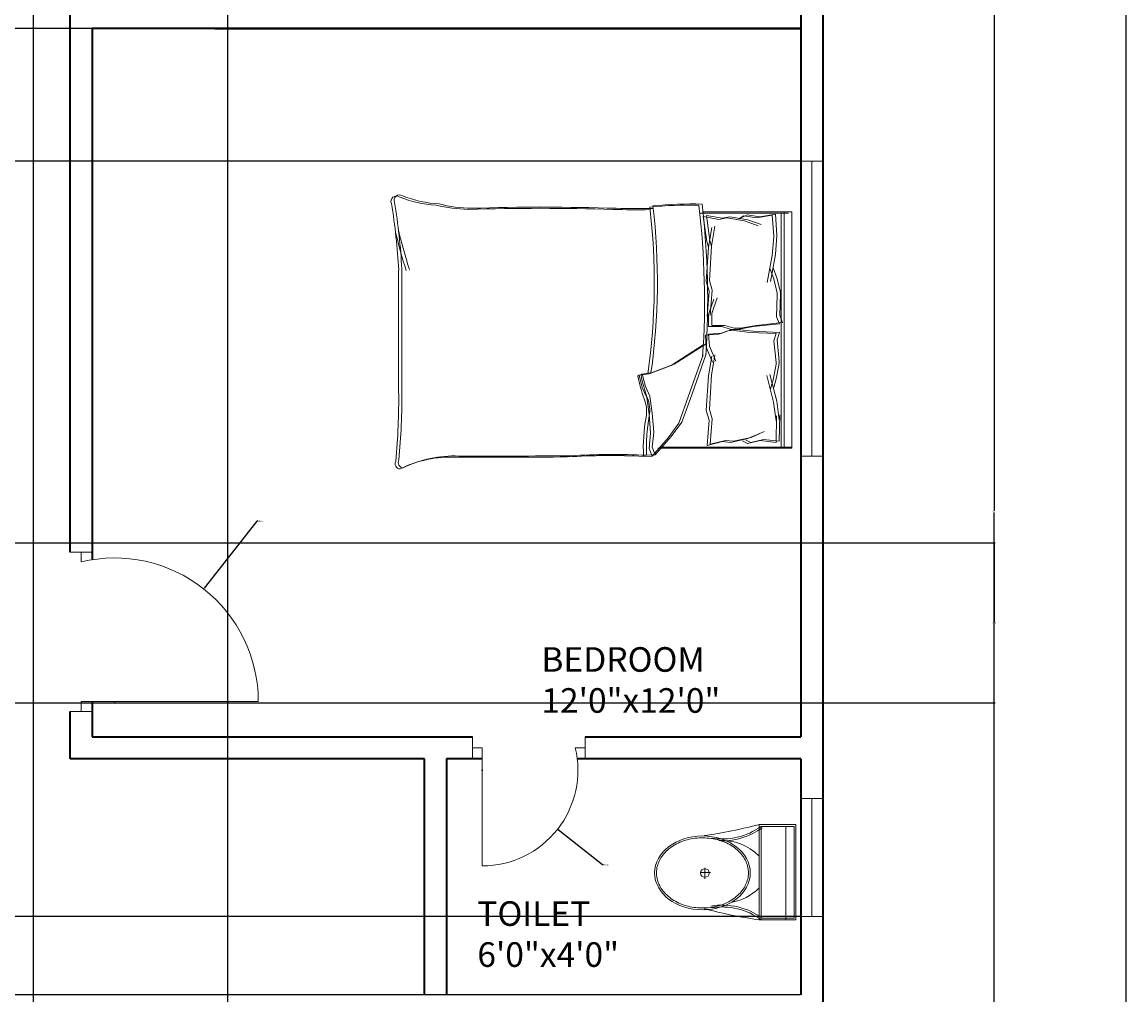
# Model space of a CAD drawing. Units: inches. Extents: x 1861 to 2564, y 1482 to 2317.
# Tile 9 of 11: x 2339 to 2564, y 1853 to 2051. Entities that reach past the tile are written whole.
import ezdxf

# ---------------------------------------------------------------- set-up
doc = ezdxf.new("R2010")
doc.units = ezdxf.units.IN
for name, color, linetype, lineweight in [('A-ANNO-DIMS', 2, 'Continuous', 18), ('A-ANNO-TTLB', 7, 'Continuous', 25), ('A-AREA-IDEN', 7, 'Continuous', 18), ('A-DOOR', 3, 'Continuous', 18), ('A-FLOR-FIXT', 8, 'Continuous', 18), ('A-FURN', 8, 'Continuous', 13), ('A-GLAZ', 4, 'Continuous', 18), ('A-WALL', 7, 'Continuous', 35)]:
    doc.layers.add(name, color=color, linetype=linetype, lineweight=lineweight)
doc.styles.get("Standard").update_dxf_attribs({"font": 'arial.ttf'})
doc.dimstyles.get("Standard").update_dxf_attribs({"dimtxt": 0.18, "dimasz": 0.18, "dimexe": 0.18, "dimexo": 0.0625, "dimgap": 0.09, "dimtad": 0, "dimtih": 1, "dimtoh": 1, "dimdec": 4, "dimzin": 0, "dimdsep": 46, "dimtxsty": 'Standard', "dimcen": 0.09, "dimadec": 0, "dimazin": 0, "dimtfac": 1, "dimtdec": 4, "dimtofl": 0, "dimtmove": 0, "dimatfit": 3, "dimfxl": 1, "dimtolj": 1, "dimtzin": 0, "dimarcsym": 0})

# ---------------------------------------------------------------- blocks, each defined once
blk = doc.blocks.new('A$C31115884')
for p, q in [((283.1, 497.7), (223.4, 497.7)), ((257.5, 466.4), (257.5, 523.2)), ((0, 200), (0, 0)), ((520, 200), (0, 200)), ((10, 190), (10, 10)), ((510, 190), (10, 190)), ((510, 10), (510, 190)), ((520, 0), (520, 200)), ((510, 54.5), (0, 54.5)), ((10, 10), (510, 10)), ((0, 0), (520, 0))]:
    blk.add_line(p, q)
blk.add_circle((255.6, 496.4), 23.6)
for centre, radius, start, end in [((2777.7, -204.6), 2807, 165.4549, 171.71327), ((3237, 905), 2807, 188.28673, 194.5451), ((-294.5, 403.3), 364.7, 324.20913, 9.34987), ((-294.5, 403.3), 374.7, 324.20913, 9.34987), ((805.8, 403.3), 364.7, 170.65013, 215.79087), ((139.5, 406.2), 293.5, 315.84364, 2.65635), ((805.8, 403.3), 374.7, 179.20365, 215.79087), ((383.6, 406.2), 293.5, 190.27735, 224.15636)]:
    blk.add_arc(centre, radius, start, end)
blk.add_ellipse((256.2, 509.9), major_axis=(0, -260.7), ratio=0.772727)
blk.add_open_spline([(256.2, 259.2), (263.1, 259.2), (270, 259.7), (287.8, 262.3), (298.7, 265.1), (319.9, 273.1), (330.2, 278.4), (350.1, 291.1), (359.7, 298.7), (377.7, 315.9), (386.2, 325.5), (401.7, 346.6), (408.8, 358.1), (421.3, 382.5), (426.8, 395.5), (435.9, 422.4), (439.5, 436.4), (444.8, 465.1), (446.5, 479.7), (447.9, 509.2), (447.6, 524), (445, 553.3), (442.7, 567.8), (436.3, 596), (432.1, 609.7), (421.9, 636), (416, 648.6), (402.5, 672.1), (395, 683), (378.6, 703), (369.8, 712.1), (351.1, 728), (341.3, 734.8), (320.9, 746.2), (310.4, 750.7), (288.9, 757.3), (278, 759.4), (256, 761), (245, 760.6), (223.1, 757.2), (212.3, 754.3), (191.1, 746.1), (180.8, 740.7), (160.9, 727.8), (151.4, 720.1), (133.5, 702.7), (125.1, 693), (109.6, 671.7), (102.6, 660.2), (90.2, 635.7), (84.9, 622.7), (76, 595.6), (72.4, 581.6), (67.2, 552.9), (65.6, 538.2), (64.4, 508.8), (64.8, 494), (67.5, 464.7), (69.9, 450.2), (76.6, 422), (80.8, 408.3), (91.1, 382.2), (97.2, 369.7), (110.8, 346.3), (118.4, 335.4), (134.8, 315.6), (143.7, 306.7), (162.4, 290.9), (172.3, 284.2), (192.8, 273), (203.3, 268.6), (224.8, 262.2), (235.8, 260.2), (249.9, 259.3), (253, 259.2), (256.2, 259.2)], degree=3, knots=[0, 0, 0, 0, 0.110105, 0.110105, 0.285049, 0.285049, 0.459994, 0.459994, 0.634938, 0.634938, 0.809882, 0.809882, 0.984827, 0.984827, 1.159771, 1.159771, 1.334715, 1.334715, 1.50966, 1.50966, 1.684604, 1.684604, 1.859549, 1.859549, 2.034493, 2.034493, 2.209437, 2.209437, 2.384382, 2.384382, 2.559326, 2.559326, 2.73427, 2.73427, 2.909215, 2.909215, 3.084159, 3.084159, 3.259103, 3.259103, 3.434048, 3.434048, 3.608992, 3.608992, 3.783936, 3.783936, 3.958881, 3.958881, 4.133825, 4.133825, 4.30877, 4.30877, 4.483714, 4.483714, 4.658658, 4.658658, 4.833603, 4.833603, 5.008547, 5.008547, 5.183491, 5.183491, 5.358436, 5.358436, 5.53338, 5.53338, 5.708324, 5.708324, 5.883269, 5.883269, 6.058213, 6.058213, 6.233158, 6.233158, 6.283185, 6.283185, 6.283185, 6.283185])
blk = doc.blocks.new('WIN-24IN')
for p, q in [((0, 24), (4.5, 24)), ((4.5, 24), (2.25, 24)), ((2.25, 24), (2.25, 0)), ((2.25, 0), (0, 0)), ((0, 0), (4.5, 0))]:
    blk.add_line(p, q)
blk = doc.blocks.new('WIN-60IN')
for p, q in [((0, 4.5), (0, 0)), ((60, 2.25), (60, 4.5)), ((60, 4.5), (60, 0)), ((0, 0), (0, 2.25)), ((0, 2.25), (60, 2.25))]:
    blk.add_line(p, q)
blk = doc.blocks.new('BED-DOUBLE')
for p, q in [((3.48, 63.34), (3.48, 81.45)), ((3.48, 63.34), (3.48, 81.45)), ((51.27, 81.45), (3.48, 81.45)), ((3.7, 62.7), (3.7, 80.81)), ((3.7, 62.7), (3.7, 80.81)), ((51.27, 81.45), (51.27, 54.84)), ((51.27, 81.45), (51.27, 54.84)), ((51.27, 81.45), (51.49, 81.45)), ((51.49, 81.45), (51.49, 80.81)), ((51.49, 80.81), (51.49, 54.2)), ((51.49, 80.81), (51.49, 54.2)), ((3.48, 79.91), (51.27, 79.91)), ((3.48, 79.91), (51.27, 79.91)), ((3.7, 79.27), (51.49, 79.27)), ((3.7, 79.27), (51.49, 79.27)), ((16.88, 78.42), (19.77, 79.14)), ((16.88, 78.42), (19.77, 79.14)), ((19.77, 79.14), (20.09, 79.14)), ((19.77, 79.14), (20.09, 79.14)), ((20.09, 79.14), (24.54, 79)), ((20.09, 79.14), (24.54, 79)), ((24.54, 79), (25.98, 79.58)), ((24.54, 79), (25.98, 79.58)), ((24.77, 78.36), (26.21, 78.94)), ((24.77, 78.36), (26.21, 78.94)), ((25.98, 79.58), (26.56, 74.23)), ((25.98, 79.58), (26.56, 74.23)), ((26.21, 78.94), (26.79, 73.59)), ((26.21, 78.94), (26.79, 73.59)), ((27.98, 78.95), (27.73, 73.58)), ((27.98, 78.95), (27.73, 73.58)), ((29.46, 78.47), (27.98, 78.95)), ((29.46, 78.47), (27.98, 78.95)), ((33.88, 78.89), (29.46, 78.47)), ((33.88, 78.89), (29.46, 78.47)), ((34.21, 78.91), (33.88, 78.89)), ((34.21, 78.91), (33.88, 78.89)), ((37.14, 78.37), (34.21, 78.91)), ((37.14, 78.37), (34.21, 78.91)), ((45.71, 78.9), (41.92, 78.38)), ((45.71, 78.9), (41.92, 78.38)), ((50.11, 78.89), (44.71, 78.99)), ((44.71, 78.99), (45.71, 78.9)), ((50.11, 78.89), (44.71, 78.99)), ((44.71, 78.99), (45.71, 78.9)), ((50.11, 78.89), (49.73, 75.68)), ((50.11, 78.89), (49.73, 75.68)), ((3.9, 78.11), (8.18, 78.44)), ((3.9, 78.11), (8.18, 78.44)), ((3.9, 78.13), (4.47, 74.95)), ((3.9, 78.13), (4.47, 74.95)), ((4.12, 77.49), (4.7, 74.31)), ((4.12, 77.49), (4.7, 74.31)), ((4.13, 77.47), (8.41, 77.8)), ((4.13, 77.47), (8.41, 77.8)), ((8.18, 78.44), (8.29, 78.42)), ((8.18, 78.44), (8.29, 78.42)), ((8.29, 78.42), (12.11, 78.13)), ((8.29, 78.42), (12.11, 78.13)), ((8.41, 77.8), (8.51, 77.78)), ((8.41, 77.8), (8.51, 77.78)), ((8.51, 77.78), (12.34, 77.49)), ((8.51, 77.78), (12.34, 77.49)), ((12.11, 78.13), (17.6, 77.12)), ((12.11, 78.13), (17.6, 77.12)), ((12.34, 77.49), (17.83, 76.48)), ((12.34, 77.49), (17.83, 76.48)), ((14.86, 77.7), (16.88, 78.42)), ((14.86, 77.7), (16.88, 78.42)), ((15.08, 77.06), (17.11, 77.78)), ((15.08, 77.06), (17.11, 77.78)), ((17.11, 77.78), (20, 78.5)), ((17.11, 77.78), (20, 78.5)), ((20, 78.5), (20.32, 78.5)), ((20, 78.5), (20.32, 78.5)), ((20.32, 78.5), (24.77, 78.36)), ((20.32, 78.5), (24.77, 78.36)), ((28.21, 78.31), (27.96, 72.94)), ((28.21, 78.31), (27.96, 72.94)), ((29.69, 77.83), (28.21, 78.31)), ((29.68, 77.83), (28.21, 78.31)), ((34.11, 78.25), (29.68, 77.83)), ((34.11, 78.25), (29.69, 77.83)), ((34.43, 78.27), (34.11, 78.25)), ((34.43, 78.27), (34.11, 78.25)), ((37.36, 77.73), (34.43, 78.27)), ((37.36, 77.73), (34.43, 78.27)), ((41.92, 78.38), (36.5, 77.02)), ((41.92, 78.38), (36.5, 77.02)), ((42.14, 77.74), (36.72, 76.38)), ((42.14, 77.74), (36.72, 76.38)), ((39.2, 77.77), (37.14, 78.37)), ((39.2, 77.77), (37.14, 78.37)), ((39.43, 77.13), (37.36, 77.73)), ((39.43, 77.13), (37.36, 77.73)), ((45.94, 78.26), (42.14, 77.74)), ((45.94, 78.26), (42.14, 77.74)), ((50.34, 78.25), (44.94, 78.35)), ((44.94, 78.35), (45.94, 78.26)), ((50.34, 78.25), (44.94, 78.35)), ((44.94, 78.35), (45.94, 78.26)), ((50.34, 78.25), (49.96, 75.04)), ((50.34, 78.25), (49.96, 75.04)), ((4.47, 74.95), (4.04, 72.35)), ((4.47, 74.95), (4.04, 72.35)), ((4.7, 74.31), (4.27, 71.71)), ((4.7, 74.31), (4.27, 71.71)), ((5.05, 72.49), (6.06, 75.24)), ((5.05, 72.49), (6.06, 75.24)), ((5.28, 71.85), (6.29, 74.6)), ((5.28, 71.85), (6.29, 74.6)), ((26.56, 74.23), (27.14, 71.04)), ((26.56, 74.23), (27.14, 71.04)), ((49.31, 73.19), (48.13, 75.87)), ((49.31, 73.19), (48.13, 75.87)), ((49.54, 72.55), (48.36, 75.23)), ((49.54, 72.55), (48.36, 75.23)), ((49.73, 75.68), (50.33, 73.11)), ((49.73, 75.68), (50.33, 73.11)), ((49.96, 75.04), (50.56, 72.47)), ((49.96, 75.04), (50.56, 72.47)), ((4.04, 72.35), (4.62, 71.33)), ((4.04, 72.35), (4.62, 71.33)), ((4.47, 68.88), (5.05, 72.49)), ((4.47, 68.88), (5.05, 72.49)), ((4.7, 68.24), (5.28, 71.85)), ((4.7, 68.24), (5.28, 71.85)), ((26.79, 73.59), (27.37, 70.41)), ((26.79, 73.59), (27.37, 70.41)), ((27.73, 73.58), (27.36, 70.37)), ((27.73, 73.58), (27.36, 70.37)), ((27.96, 72.94), (27.58, 69.73)), ((27.96, 72.94), (27.58, 69.73)), ((50.11, 69.62), (49.31, 73.19)), ((50.11, 69.62), (49.31, 73.19)), ((50.34, 68.98), (49.54, 72.55)), ((50.34, 68.98), (49.54, 72.55)), ((50.33, 73.11), (49.82, 72.06)), ((50.33, 73.11), (49.82, 72.06)), ((50.56, 72.47), (50.04, 71.42)), ((50.56, 72.47), (50.04, 71.42)), ((4.27, 71.71), (4.85, 70.69)), ((4.27, 71.71), (4.85, 70.69)), ((27.14, 69.74), (26.56, 67.86)), ((27.14, 69.74), (26.56, 67.86)), ((27.14, 71.04), (27.14, 69.74)), ((27.14, 71.04), (27.14, 69.74)), ((27.36, 70.37), (27.44, 69.07)), ((27.36, 70.37), (27.44, 69.07)), ((27.37, 70.41), (27.37, 69.1)), ((27.37, 70.41), (27.37, 69.1)), ((27.58, 69.73), (27.67, 68.43)), ((27.58, 69.73), (27.67, 68.43)), ((49.92, 68.01), (50.11, 69.62)), ((49.92, 68.01), (50.11, 69.62)), ((4.76, 67.29), (4.47, 68.88)), ((4.76, 67.29), (4.47, 68.88)), ((4.99, 66.65), (4.7, 68.24)), ((4.99, 66.65), (4.7, 68.24)), ((26.56, 67.86), (26.56, 65.18)), ((26.56, 67.86), (26.56, 65.18)), ((27.37, 69.1), (26.79, 67.22)), ((27.37, 69.1), (26.79, 67.22)), ((27.44, 69.07), (28.13, 67.23)), ((27.44, 69.07), (28.13, 67.23)), ((27.67, 68.43), (28.36, 66.59)), ((27.67, 68.43), (28.36, 66.59)), ((50.7, 64.87), (49.92, 68.01)), ((50.7, 64.87), (49.92, 68.01)), ((50.15, 67.37), (50.34, 68.98)), ((50.15, 67.37), (50.34, 68.98)), ((50.93, 64.23), (50.15, 67.37)), ((50.93, 64.23), (50.15, 67.37)), ((4.18, 64.1), (4.76, 67.29)), ((4.18, 64.1), (4.76, 67.29)), ((4.41, 63.46), (4.99, 66.65)), ((4.41, 63.46), (4.99, 66.65)), ((6.38, 65.82), (10.41, 65.15)), ((6.38, 65.82), (10.41, 65.15)), ((6.61, 65.18), (10.64, 64.51)), ((6.61, 65.18), (10.64, 64.51)), ((10.41, 65.15), (9.28, 64.83)), ((10.41, 65.15), (9.28, 64.83)), ((10.41, 65.15), (17.42, 64.72)), ((10.41, 65.15), (17.42, 64.72)), ((17.42, 64.72), (19.38, 65.28)), ((17.42, 64.72), (19.38, 65.28)), ((19.38, 65.28), (24.52, 64.87)), ((19.38, 65.28), (24.52, 64.87)), ((24.1, 65.18), (20.96, 66.27)), ((24.1, 65.18), (20.96, 66.27)), ((24.33, 64.54), (21.19, 65.63)), ((24.33, 64.54), (21.19, 65.63)), ((26.56, 65.18), (24.1, 65.18)), ((26.56, 65.18), (24.1, 65.18)), ((26.79, 67.22), (26.79, 64.54)), ((26.79, 67.22), (26.79, 64.54)), ((28.13, 67.23), (28.3, 64.55)), ((28.13, 67.23), (28.3, 64.55)), ((28.36, 66.59), (28.53, 63.91)), ((28.36, 66.59), (28.53, 63.91)), ((30.75, 64.71), (33.82, 65.99)), ((30.75, 64.71), (33.82, 65.99)), ((30.98, 64.07), (34.05, 65.35)), ((30.98, 64.07), (34.05, 65.35)), ((32.56, 65.82), (36.6, 65.15)), ((32.57, 65.82), (36.6, 65.15)), ((32.79, 65.18), (36.83, 64.51)), ((32.79, 65.18), (36.83, 64.51)), ((36.6, 65.15), (43.61, 64.72)), ((36.6, 65.15), (43.61, 64.72)), ((43.61, 64.72), (45.57, 65.28)), ((43.61, 64.72), (45.57, 65.28)), ((45.57, 65.28), (50.7, 64.87)), ((45.57, 65.28), (50.7, 64.87)), ((9.28, 64.83), (4.18, 64.1)), ((9.28, 64.83), (4.18, 64.1)), ((9.51, 64.19), (4.41, 63.46)), ((9.51, 64.19), (4.41, 63.46)), ((10.64, 64.51), (9.51, 64.19)), ((10.64, 64.51), (9.51, 64.19)), ((10.64, 64.51), (17.65, 64.08)), ((10.64, 64.51), (17.65, 64.08)), ((17.65, 64.08), (19.61, 64.64)), ((17.65, 64.08), (19.61, 64.64)), ((19.61, 64.64), (24.75, 64.23)), ((19.61, 64.64), (24.74, 64.23)), ((26.79, 64.54), (24.33, 64.54)), ((26.79, 64.54), (24.33, 64.54)), ((28.3, 64.55), (30.75, 64.71)), ((28.3, 64.55), (30.75, 64.71)), ((28.53, 63.91), (30.98, 64.07)), ((28.53, 63.91), (30.98, 64.07)), ((30.26, 64.06), (34.45, 57.57)), ((30.26, 64.06), (34.45, 57.57)), ((30.49, 63.42), (34.68, 56.93)), ((30.49, 63.42), (34.68, 56.93)), ((40.65, 61.13), (32.31, 64.06)), ((40.64, 61.13), (32.31, 64.06)), ((40.87, 60.49), (32.54, 63.42)), ((40.87, 60.49), (32.54, 63.42)), ((36.83, 64.51), (43.84, 64.08)), ((36.83, 64.51), (43.84, 64.08)), ((43.84, 64.08), (45.8, 64.64)), ((43.84, 64.08), (45.8, 64.64)), ((45.8, 64.64), (50.93, 64.23)), ((45.8, 64.64), (50.93, 64.23)), ((46.22, 59.12), (40.64, 61.13)), ((46.22, 59.12), (40.65, 61.13)), ((46.45, 58.48), (40.87, 60.49)), ((46.45, 58.48), (40.87, 60.49)), ((49.16, 56.95), (46.22, 59.12)), ((49.16, 56.95), (46.22, 59.12)), ((49.39, 56.31), (46.45, 58.48)), ((49.39, 56.31), (46.45, 58.48)), ((34.45, 57.57), (36.15, 53.08)), ((34.45, 57.57), (36.15, 53.08)), ((34.68, 56.93), (36.38, 52.44)), ((34.68, 56.93), (36.38, 52.44)), ((52.87, 53.7), (49.16, 56.95)), ((52.87, 53.7), (49.16, 56.95)), ((53.1, 53.06), (49.39, 56.31)), ((53.1, 53.06), (49.39, 56.31)), ((36.15, 53.08), (36.46, 51.07)), ((36.15, 53.08), (36.46, 51.07)), ((36.38, 52.44), (36.69, 50.43)), ((36.38, 52.44), (36.69, 50.43)), ((36.46, 51.07), (38.94, 51.69)), ((36.46, 51.07), (38.94, 51.69)), ((38.94, 51.69), (40.95, 52.62)), ((38.94, 51.69), (40.95, 52.62)), ((39.17, 51.05), (41.18, 51.98)), ((39.17, 51.05), (41.18, 51.98)), ((40.95, 52.62), (44.36, 53.08)), ((40.95, 52.62), (44.36, 53.08)), ((41.18, 51.98), (44.59, 52.44)), ((41.18, 51.98), (44.59, 52.44)), ((44.36, 53.08), (48.23, 53.39)), ((44.36, 53.08), (48.23, 53.39)), ((44.59, 52.44), (48.46, 52.75)), ((44.59, 52.44), (48.46, 52.75)), ((48.23, 53.39), (51.33, 53.08)), ((48.23, 53.39), (51.33, 53.08)), ((48.46, 52.75), (51.56, 52.44)), ((48.46, 52.75), (51.56, 52.44)), ((51.33, 53.08), (52.87, 53.7)), ((51.33, 53.08), (52.87, 53.7)), ((51.56, 52.44), (53.1, 53.06)), ((51.56, 52.44), (53.1, 53.06)), ((52.95, 51.95), (52.87, 53.7, 3.87)), ((52.95, 51.95), (52.87, 53.7, 3.87)), ((53.18, 51.32), (53.1, 53.06, 3.87)), ((53.18, 51.32), (53.1, 53.06, 3.87)), ((36.69, 50.43), (39.17, 51.05)), ((36.69, 50.43), (39.17, 51.05)), ((15.06, 2.2), (39.68, 2.2)), ((15.06, 2.2), (39.68, 2.2)), ((15.29, 1.56), (39.91, 1.56)), ((15.29, 1.56), (39.91, 1.56))]:
    blk.add_line(p, q)
for centre, radius, start, end in [((85.16, 61.35), 83.31, 178.7218, 185.604), ((85.16, 61.35), 83.31, 178.7218, 185.604), ((21.36, -100.61), 164.97, 86.0865, 96.7821), ((21.36, -100.61), 164.97, 86.0865, 96.7821), ((21.59, -101.25), 164.97, 86.0865, 96.7821), ((21.59, -101.25), 164.97, 86.0865, 96.7821), ((85.39, 60.71), 83.31, 178.7218, 185.604), ((85.39, 60.71), 83.31, 178.7218, 185.604), ((17.76, -74.87), 129.02, 81.7845, 96.9006), ((17.76, -74.87), 129.02, 81.7845, 96.9006), ((17.99, -75.51), 129.02, 81.7845, 96.9006), ((17.98, -75.51), 129.02, 81.7845, 96.9006), ((-167.31, 50.27), 170.11, 358.4762, 1.0082), ((-167.31, 50.27), 170.11, 358.4762, 1.0082), ((-167.08, 49.63), 170.11, 358.4762, 1.0082), ((-167.08, 49.63), 170.11, 358.4762, 1.0082), ((31.15, 79.96), 29.65, 280.6617, 289.8806), ((31.15, 79.96), 29.65, 280.6617, 289.8806), ((43.74, 46.38), 6.22, 78.6608, 113.7384), ((43.74, 46.38), 6.22, 78.6608, 113.7384), ((43.97, 45.74), 6.22, 78.6608, 113.7384), ((43.97, 45.74), 6.22, 78.6608, 113.7384), ((51.33, 88.1), 36.18, 259.8763, 272.5657), ((51.33, 88.1), 36.18, 259.8763, 272.5657), ((51.56, 87.46), 36.18, 259.8763, 272.5657), ((51.56, 87.46), 36.18, 259.8763, 272.5657), ((182.27, 45.13), 129.5, 176.9791, 183.8365), ((182.27, 45.13), 129.5, 176.9791, 183.8365), ((36.64, 51.01), 0.185, 160.2464, 271.1377), ((36.64, 51.01), 0.185, 160.2464, 271.1377), ((36.87, 50.37), 0.185, 160.2464, 271.1377), ((36.87, 50.37), 0.185, 160.2464, 271.1377), ((31.38, 79.32), 29.65, 280.6617, 289.8806), ((31.38, 79.32), 29.65, 280.6617, 289.8806), ((182.5, 44.49), 129.5, 176.9791, 183.8365), ((182.49, 44.49), 129.5, 176.9791, 183.8365), ((484.82, 30.83), 482.31, 178.2277, 181.7185), ((484.82, 30.83), 482.31, 178.2277, 181.7185), ((485.05, 30.19), 482.31, 178.2277, 181.7185), ((485.05, 30.19), 482.31, 178.2277, 181.7185), ((-4508.74, 13.62), 4561.86, 0.00217, 0.28689), ((-4508.74, 13.62), 4561.86, 0.00217, 0.28689), ((-4508.51, 12.98), 4561.86, 0.00217, 0.28689), ((-4508.51, 12.98), 4561.86, 0.00217, 0.28689), ((-26.9, 16.93), 29.63, 346.0648, 358.9113), ((-26.9, 16.93), 29.63, 346.0648, 358.9113), ((-26.67, 16.29), 29.63, 346.0648, 358.9113), ((-26.67, 16.29), 29.63, 346.0648, 358.9113), ((76.16, 12.78), 23.07, 177.4714, 206.4681), ((76.16, 12.78), 23.07, 177.4714, 206.4681), ((76.39, 12.14), 23.07, 177.4714, 206.4681), ((76.39, 12.14), 23.07, 177.4714, 206.4681), ((-21.66, 11.17), 23.56, 337.9751, 356.652), ((-21.66, 11.17), 23.56, 337.9751, 356.652), ((-21.43, 10.53), 23.56, 337.9751, 356.652), ((-21.43, 10.53), 23.56, 337.9751, 356.652), ((1.09, 1.73), 1.09, 146.1736, 293.4781), ((1.09, 1.73), 1.09, 146.1736, 293.4781), ((-17.22, 105.16), 106.46, 283.3832, 287.7053), ((-17.22, 105.16), 106.46, 283.3832, 287.7053), ((-16.99, 104.52), 106.46, 283.3832, 287.7053), ((-16.99, 104.52), 106.46, 283.3832, 287.7053), ((54.41, 2.58), 1.1, 242.6588, 356.02), ((54.41, 2.58), 1.1, 242.6588, 356.02), ((1.32, 1.09), 1.09, 146.1736, 293.4781), ((1.32, 1.09), 1.09, 146.1736, 293.4781), ((21.43, -119.39), 121.76, 92.9958, 99.4091), ((21.43, -119.39), 121.76, 92.9958, 99.4091), ((21.66, -120.03), 121.76, 92.9958, 99.4091), ((21.66, -120.03), 121.76, 92.9958, 99.4091), ((41.15, -130.83), 133.04, 84.4998, 90.6351), ((41.15, -130.83), 133.04, 84.4998, 90.6351), ((41.38, -131.47), 133.04, 84.4998, 90.6351), ((41.38, -131.47), 133.04, 84.4998, 90.6351), ((54.64, 1.94), 1.1, 242.6588, 356.02), ((54.64, 1.94), 1.1, 242.6588, 356.02)]:
    blk.add_arc(centre, radius, start, end)
blk = doc.blocks.new('*D38')
at = {"layer": 'A-ANNO-DIMS', "color": 0, "lineweight": -2, "transparency": 16777216}
for p, q in [((2341.74, 2250.82), (2341.74, 1545.6)), ((2381.24, 2250.82), (2381.24, 1545.6)), ((2341.92, 1545.78), (2361.16, 1545.78)), ((2381.06, 1545.78), (2361.81, 1545.78))]:
    blk.add_line(p, q, dxfattribs=at)
at = {"layer": 'A-ANNO-DIMS', "color": 0, "transparency": 16777216}
for points in [[(2341.92, 1545.81), (2341.92, 1545.75), (2341.74, 1545.78)], [(2381.06, 1545.81), (2381.06, 1545.75), (2381.24, 1545.78)]]:
    blk.add_solid(points, dxfattribs=at)
at = {"layer": 'Defpoints', "color": 0, "transparency": 16777216}
for p in [(2341.74, 2250.89), (2381.24, 2250.89), (2381.24, 1545.78)]:
    blk.add_point(p, dxfattribs=at)
at = {"layer": 'A-ANNO-DIMS', "color": 0, "transparency": 16777216, "insert": (2361.49, 1545.78), "char_height": 0.18, "attachment_point": 5}
blk.add_mtext('\\A1;39.5', dxfattribs=at)
blk = doc.blocks.new('*D45')
at = {"layer": 'A-ANNO-DIMS', "color": 0, "lineweight": -2, "transparency": 16777216}
for p, q in [((2502.3, 2255.39), (2537.22, 2255.39)), ((2537.04, 2255.21), (2537.04, 1951.82)), ((2537.04, 1648.07), (2537.04, 1951.45)), ((2473.32, 1647.89), (2537.22, 1647.89))]:
    blk.add_line(p, q, dxfattribs=at)
at = {"layer": 'A-ANNO-DIMS', "color": 0, "transparency": 16777216}
for points in [[(2537.01, 2255.21), (2537.07, 2255.21), (2537.04, 2255.39)], [(2537.01, 1648.07), (2537.07, 1648.07), (2537.04, 1647.89)]]:
    blk.add_solid(points, dxfattribs=at)
at = {"layer": 'Defpoints', "color": 0, "transparency": 16777216}
for p in [(2502.24, 2255.39), (2537.04, 2255.39), (2473.26, 1647.89)]:
    blk.add_point(p, dxfattribs=at)
at = {"layer": 'A-ANNO-DIMS', "color": 0, "transparency": 16777216, "insert": (2537.04, 1951.64), "char_height": 0.18, "attachment_point": 5}
blk.add_mtext('\\A1;607.5', dxfattribs=at)
blk = doc.blocks.new('*D53')
at = {"layer": 'A-ANNO-DIMS', "color": 0, "lineweight": -2, "transparency": 16777216}
for p, q in [((2076.3, 1945.29), (2537.22, 1945.29)), ((2537.04, 1945.11), (2537.04, 1929.2)), ((2537.04, 1912.93), (2537.04, 1928.84)), ((2076.3, 1912.75), (2537.22, 1912.75))]:
    blk.add_line(p, q, dxfattribs=at)
at = {"layer": 'A-ANNO-DIMS', "color": 0, "transparency": 16777216}
for points in [[(2537.01, 1945.11), (2537.07, 1945.11), (2537.04, 1945.29)], [(2537.01, 1912.93), (2537.07, 1912.93), (2537.04, 1912.75)]]:
    blk.add_solid(points, dxfattribs=at)
at = {"layer": 'Defpoints', "color": 0, "transparency": 16777216}
for p in [(2076.24, 1945.29), (2537.04, 1945.29), (2076.24, 1912.75)]:
    blk.add_point(p, dxfattribs=at)
at = {"layer": 'A-ANNO-DIMS', "color": 0, "transparency": 16777216, "insert": (2537.04, 1929.02), "char_height": 0.18, "attachment_point": 5}
blk.add_mtext('\\A1;32.544', dxfattribs=at)
blk = doc.blocks.new('*D65')
at = {"layer": 'A-ANNO-DIMS', "color": 0, "lineweight": -2, "transparency": 16777216}
for p, q in [((2497.68, 2049.89), (1892.76, 2049.89)), ((1892.94, 2049.71), (1892.94, 2036.58)), ((1892.94, 2023.09), (1892.94, 2036.22)), ((2497.68, 2022.91), (1892.76, 2022.91))]:
    blk.add_line(p, q, dxfattribs=at)
at = {"layer": 'A-ANNO-DIMS', "color": 0, "transparency": 16777216}
for points in [[(1892.91, 2049.71), (1892.97, 2049.71), (1892.94, 2049.89)], [(1892.91, 2023.09), (1892.97, 2023.09), (1892.94, 2022.91)]]:
    blk.add_solid(points, dxfattribs=at)
at = {"layer": 'Defpoints', "color": 0, "transparency": 16777216}
for p in [(2497.74, 2049.89), (1892.94, 2022.91), (2497.74, 2022.91)]:
    blk.add_point(p, dxfattribs=at)
at = {"layer": 'A-ANNO-DIMS', "color": 0, "transparency": 16777216, "insert": (1892.94, 2036.4), "char_height": 0.18, "attachment_point": 5}
blk.add_mtext('\\A1;26.973', dxfattribs=at)
blk = doc.blocks.new('*D66')
at = {"layer": 'A-ANNO-DIMS', "color": 0, "lineweight": -2, "transparency": 16777216}
for p, q in [((2497.68, 1869.33), (1892.76, 1869.33)), ((1892.94, 1869.15), (1892.94, 1861.54)), ((1892.94, 1853.57), (1892.94, 1861.17)), ((2497.68, 1853.39), (1892.76, 1853.39))]:
    blk.add_line(p, q, dxfattribs=at)
at = {"layer": 'A-ANNO-DIMS', "color": 0, "transparency": 16777216}
for points in [[(1892.91, 1869.15), (1892.97, 1869.15), (1892.94, 1869.33)], [(1892.91, 1853.57), (1892.97, 1853.57), (1892.94, 1853.39)]]:
    blk.add_solid(points, dxfattribs=at)
at = {"layer": 'Defpoints', "color": 0, "transparency": 16777216}
for p in [(2497.74, 1869.33), (1892.94, 1853.39), (2497.74, 1853.39)]:
    blk.add_point(p, dxfattribs=at)
at = {"layer": 'A-ANNO-DIMS', "color": 0, "transparency": 16777216, "insert": (1892.94, 1861.36), "char_height": 0.18, "attachment_point": 5}
blk.add_mtext('\\A1;15.94', dxfattribs=at)
blk = doc.blocks.new('*D81')
at = {"layer": 'A-ANNO-DIMS', "color": 0, "lineweight": -2, "transparency": 16777216}
for p, q in [((2387.21, 1949.71), (2376.48, 1936.1)), ((2387.39, 1949.71), (2387.21, 1949.71)), ((2358.21, 1913.04), (2358.39, 1913.04)), ((2358.3, 1912.95), (2358.3, 1913.13))]:
    blk.add_line(p, q, dxfattribs=at)
at = {"layer": 'A-ANNO-DIMS', "color": 0, "transparency": 16777216}
blk.add_solid([(2376.46, 1936.12), (2376.51, 1936.08), (2376.37, 1935.96)], dxfattribs=at)
at = {"layer": 'Defpoints', "color": 0, "transparency": 16777216}
for p in [(2376.37, 1935.96), (2358.3, 1913.04)]:
    blk.add_point(p, dxfattribs=at)
at = {"layer": 'A-ANNO-DIMS', "color": 0, "transparency": 16777216, "insert": (2387.94, 1949.71), "char_height": 0.18, "attachment_point": 5}
blk.add_mtext('\\A1;R29.186', dxfattribs=at)
blk = doc.blocks.new('*D87')
at = {"layer": 'A-ANNO-DIMS', "color": 0, "lineweight": -2, "transparency": 16777216}
for p, q in [((2432.92, 1899.07), (2433.1, 1899.07)), ((2433.01, 1898.98), (2433.01, 1899.16)), ((2457.44, 1879.84), (2448.42, 1886.94)), ((2457.62, 1879.84), (2457.44, 1879.84))]:
    blk.add_line(p, q, dxfattribs=at)
at = {"layer": 'A-ANNO-DIMS', "color": 0, "transparency": 16777216}
blk.add_solid([(2448.44, 1886.96), (2448.4, 1886.92), (2448.28, 1887.05)], dxfattribs=at)
at = {"layer": 'Defpoints', "color": 0, "transparency": 16777216}
for p in [(2433.01, 1899.07), (2448.28, 1887.05)]:
    blk.add_point(p, dxfattribs=at)
at = {"layer": 'A-ANNO-DIMS', "color": 0, "transparency": 16777216, "insert": (2458.17, 1879.84), "char_height": 0.18, "attachment_point": 5}
blk.add_mtext('\\A1;R19.436', dxfattribs=at)

msp = doc.modelspace()

# ---------------------------------------------------------------- linework, layer by layer
at = {"layer": 'A-ANNO-TTLB'}
msp.add_lwpolyline([(1861.1332, 2316.6589), (2563.8077, 2316.6589), (2563.8077, 1482.0728), (1861.1332, 1482.0728)], close=True, dxfattribs=at)
at = {"layer": 'A-DOOR'}
for p, q in [((2349.2393, 1943.42), (2353.7393, 1943.42)), ((2353.7393, 1943.42), (2349.2393, 1943.42)), ((2349.2393, 1943.42), (2351.4893, 1943.42)), ((2351.4893, 1943.42), (2351.4893, 1941.42)), ((2351.4893, 1911.04), (2351.4893, 1913.04)), ((2351.4893, 1913.04), (2387.4893, 1913.04)), ((2353.7393, 1911.04), (2349.2393, 1911.04)), ((2349.2393, 1911.04), (2351.4893, 1911.04)), ((2431.0077, 1901.3854), (2431.0077, 1905.8854)), ((2431.0077, 1905.8854), (2431.0077, 1903.6354)), ((2453.9, 1905.8854), (2453.9, 1901.3854)), ((2431.0077, 1903.6354), (2433.0077, 1903.6354)), ((2433.0077, 1903.6354), (2433.0077, 1879.6354)), ((2453.9, 1903.6354), (2451.9, 1903.6354)), ((2453.9, 1901.3854), (2453.9, 1903.6354))]:
    msp.add_line(p, q, dxfattribs=at)
for centre, radius, start, end in [((2358.3028, 1913.04), 29.1864, 360, 103.500254), ((2433.0077, 1899.0712), 19.4359, 270, 13.581687)]:
    msp.add_arc(centre, radius, start, end, dxfattribs=at)
at = {"layer": 'A-WALL'}
for p, q in [((2502.2393, 2255.3854), (2502.2393, 1700.3854)), ((2497.7393, 2102.3854), (2497.7393, 1905.8854)), ((2349.2393, 2049.8854), (2349.2393, 2054.3854)), ((2349.2393, 1943.42), (2349.2393, 2049.8854)), ((2497.7393, 2049.8854), (2353.7393, 2049.8854)), ((2353.7393, 2049.8854), (2353.7393, 1941.8675)), ((2378.6849, 2049.8854), (2497.7393, 2049.8854)), ((2353.7393, 1913.04), (2353.7393, 1905.8854)), ((2349.2393, 1901.3854), (2349.2393, 1911.04)), ((2353.7393, 1905.8854), (2431.0077, 1905.8854)), ((2453.9, 1905.8854), (2497.7393, 1905.8854)), ((2353.7393, 1901.3854), (2349.2393, 1901.3854)), ((2421.2393, 1901.3854), (2353.7393, 1901.3854)), ((2421.2393, 1853.3854), (2421.2393, 1901.3854)), ((2425.7393, 1901.3854), (2425.7393, 1853.3854)), ((2433.0077, 1901.3854), (2425.7393, 1901.3854)), ((2433.0077, 1901.3854), (2425.7393, 1901.3854)), ((2497.7393, 1901.3854), (2452.3053, 1901.3854)), ((2497.7393, 1901.3854), (2452.3053, 1901.3854)), ((2497.7393, 1901.3854), (2497.7393, 1853.3854))]:
    msp.add_line(p, q, dxfattribs=at)

# ---------------------------------------------------------------- block references
at = {"layer": 'A-FLOR-FIXT', "xscale": 0.0372717239612423, "yscale": 0.0372717239612423, "zscale": 0.0372717239612423, "rotation": 89.99999999999999}
msp.add_blockref('A$C31115884', (2496.7591, 1868.6493), dxfattribs=at)
at = {"layer": 'A-FURN', "rotation": 270}
msp.add_blockref('BED-DOUBLE', (2414.4548, 2016.0556), dxfattribs=at)
at = {"layer": 'A-GLAZ', "extrusion": (0, 0, -1), "zscale": -1, "rotation": 90}
msp.add_blockref('WIN-60IN', (-2497.7439, 1962.9137), dxfattribs=at)
at = {"layer": 'A-GLAZ', "rotation": 180}
msp.add_blockref('WIN-24IN', (2502.2385, 1893.3235), dxfattribs=at)

# ---------------------------------------------------------------- texts
at = {"layer": 'A-AREA-IDEN', "char_height": 5, "attachment_point": 1}
for s, width, insert in [('BEDROOM\\P12\'0"x12\'0"', 157.139308, (2445.0187, 1924.0885)), ('TOILET\\P6\'0"x4\'0"', 83.843436, (2432.0047, 1872.4274))]:
    msp.add_mtext_dynamic_manual_height_columns(s, width=width, gutter_width=12.5, heights=[0], dxfattribs=dict(at, insert=insert))

# ---------------------------------------------------------------- dimensions: what is measured, and where the dimension line sits
at = {"layer": 'A-ANNO-DIMS'}
for base, p1, p2, override, picture, middle in [((2537.0393, 2255.3854), (2473.2613, 1647.8854), (2502.2393, 2255.3854), {"dimdec": 1, "dimlfac": 1, "dimrnd": 0, "dimzin": 0, "dimdsep": 46, "dimlunit": 2}, '*D45', (2537.0393, 1951.6354)), ((1892.9393, 2022.9123), (2497.7393, 2049.8854), (2497.7393, 2022.9123), {"dimdec": 3, "dimlfac": 1, "dimrnd": 0, "dimzin": 0, "dimdsep": 46, "dimlunit": 2}, '*D65', (1892.9393, 2036.3989)), ((2537.0393, 1945.2921), (2076.2393, 1912.7479), (2076.2393, 1945.2921), {"dimdec": 3, "dimlfac": 1, "dimrnd": 0, "dimzin": 0, "dimdsep": 46, "dimlunit": 2}, '*D53', (2537.0393, 1929.02)), ((1892.9393, 1853.3854), (2497.7393, 1869.3266), (2497.7393, 1853.3854), {"dimdec": 2, "dimlfac": 1, "dimrnd": 0, "dimzin": 0, "dimdsep": 46, "dimlunit": 2}, '*D66', (1892.9393, 1861.356))]:
    dim = msp.add_linear_dim(base=base, p1=p1, p2=p2, angle=90, dimstyle='Standard', override=override, dxfattribs=at)
    dim.commit()
    dim.dimension.update_dxf_attribs({"geometry": picture, "text_midpoint": middle})
dim = msp.add_linear_dim(base=(2381.2368, 1545.7777), p1=(2341.7393, 2250.8854), p2=(2381.2368, 2250.8854), dimstyle='Standard', override={"dimdec": 1, "dimlfac": 1, "dimrnd": 0, "dimzin": 0, "dimdsep": 46, "dimlunit": 2}, dxfattribs=at)
dim.commit()
dim.dimension.update_dxf_attribs({"geometry": '*D38', "text_midpoint": (2361.488, 1545.7777)})
for center, mpoint, picture, middle in [((2358.30284, 1913.04003), (2376.37181, 1935.96077), '*D81', (2387.9429, 1949.71321)), ((2433.0077, 1899.0712), (2448.28, 1887.05), '*D87', (2458.173, 1879.8373))]:
    dim = msp.add_radius_dim(center=center, mpoint=mpoint, dimstyle='Standard', override={"dimdec": 3, "dimlfac": 1, "dimrnd": 0, "dimzin": 0, "dimdsep": 46, "dimlunit": 2}, dxfattribs=at)
    dim.commit()
    dim.dimension.update_dxf_attribs({"geometry": picture, "text_midpoint": middle, "dimtype": 164})

doc.saveas('drawing.dxf')
